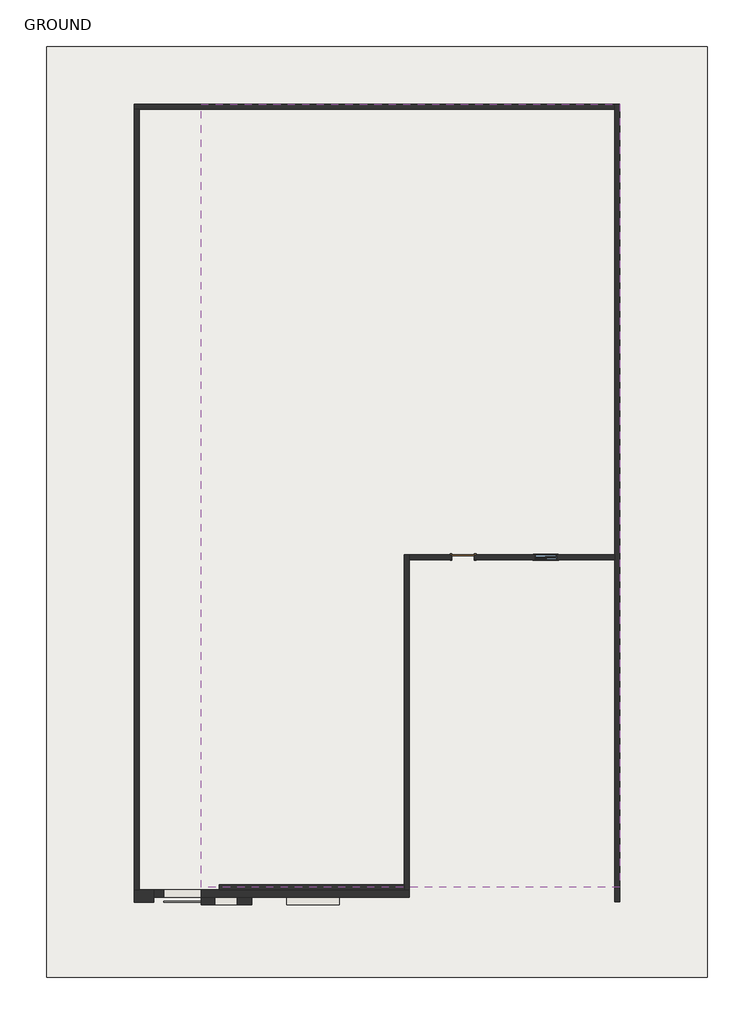
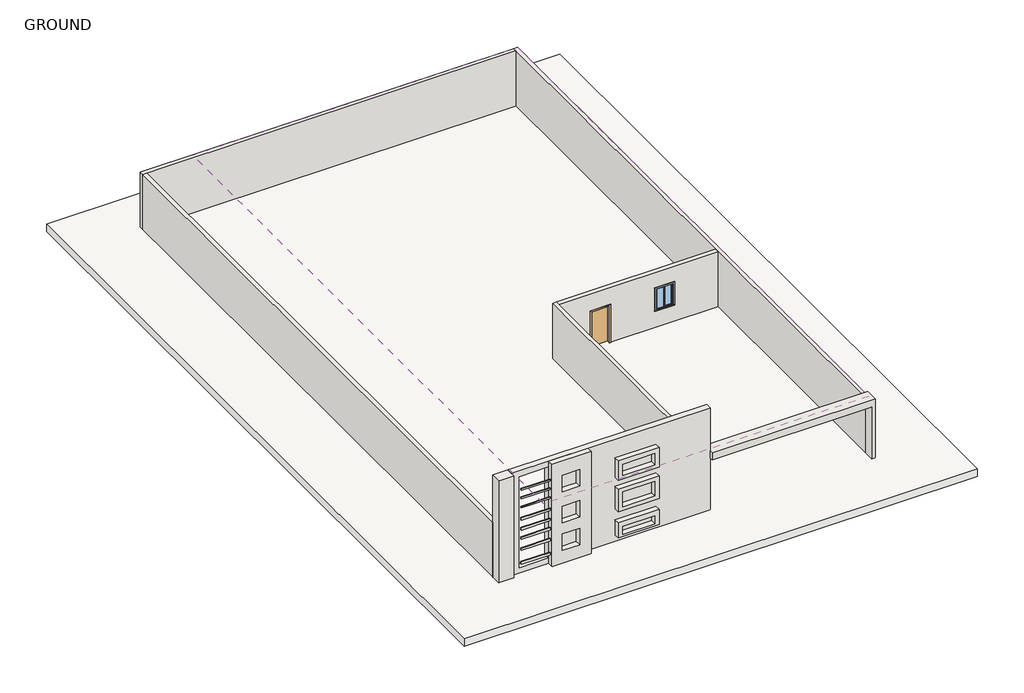
# One storey: 12 walls, 1 covering, 1 door, 1 slab, 1 window.
"""IFC4 building model written with IfcOpenShell, lengths in millimetres."""

from ifc_helpers import new_model, si_unit, frame, origin, origin_with_axes, place, context, project, spatial, polyline, outline, extrude, faceted_brep, transform, mapped, element, save
from components import m_single_flush_0915_x_2032mm_26613924, walls_2_walls_2_e7feafe1, walls_3_walls_3_a1481ceb, walls_4_walls_4_1aaea7ad, walls_5_walls_5_99fd860d, walls_6_walls_6_eefe2e9b, walls_7_walls_7_71d3a732, window_242facca

model = new_model("IFC4")

# Units and contexts
model_context = context("Model", 3, world=origin())
ifc_project = project(units=[si_unit("LENGTHUNIT", "METRE", prefix="MILLI")], contexts=[model_context])

# Site, building, storey
site = spatial("IfcSite", under=ifc_project)
building = spatial("IfcBuilding", under=site)
storey = spatial("IfcBuildingStorey", under=building, Name="GROUND", Elevation=0.0)

# Covering
placement = place(None, origin())
element("IfcCovering", 1, ObjectType="600 x 1200mm grid", at=placement, inside=storey, context=model_context, shape_type="SweptSolid", body=[
    extrude(outline(polyline([(-15779.6883357, -20030.9210337), (-15779.6883357, 11768.2789663), (1204.9616643, 11768.2789663), (1204.9616643, -20030.9210337), (-15779.6883357, -20030.9210337)])), frame((0.0, 0.0, 3048.0), z_axis=(0.0, 0.0, 1.0), x_axis=(1.0, 0.0, 0.0)), (0.0, 0.0, 1.0), 52.0),
])

# Door
m_single_flush_0915_x_2032mm_shape = m_single_flush_0915_x_2032mm_26613924(model_context)
element("IfcDoor", 2, ObjectType="M_Single-Flush : 0915 x 2032mm", at=placement, inside=storey, context=model_context, shape_type="MappedRepresentation", body=[
    mapped(m_single_flush_0915_x_2032mm_shape, transform((-5143.4383357, -6619.7210337, 0.0), x_axis=(-1.0, 0.0, 0.0), y_axis=(0.0, -1.0, 0.0), z_axis=(0.0, 0.0, 1.0))),
])

# Slab
element("IfcSlab", 3, ObjectType="Generic Floor - 400mm", at=placement, inside=storey, context=model_context, shape_type="SweptSolid", body=[
    extrude(outline(polyline([(4762.5616643, 14106.6789663), (4762.5616643, -23688.5210337), (-22059.8383357, -23688.5210337), (-22059.8383357, 14106.6789663), (4762.5616643, 14106.6789663)])), frame((0.0, 0.0, -400.0), z_axis=(0.0, 0.0, 1.0), x_axis=(1.0, 0.0, 0.0)), (0.0, 0.0, 1.0), 400.0),
])

# Walls
element("IfcWall", 4, ObjectType="Generic - 9\"", at=placement, inside=storey, context=model_context, shape_type="Brep", body=[
    faceted_brep([(-18502.2383357, 11568.2789663, 0.0), (-18302.2383357, 11568.2789663, 0.0), (1004.9616643, 11568.2789663, 0.0), (1004.9616643, 11568.2789663, 3048.0), (-18302.2383357, 11568.2789663, 3048.0), (-18502.2383357, 11568.2789663, 3048.0), (-18502.2383357, 11768.2789663, 0.0), (-18502.2383357, 11768.2789663, 3048.0), (1004.9616643, 11768.2789663, 3048.0), (1004.9616643, 11768.2789663, 0.0)], [[[0, 1, 2, 3, 4, 5]], [[6, 7, 8, 9]], [[2, 1, 0, 6, 9]], [[5, 4, 3, 8, 7]], [[0, 5, 7, 6]], [[3, 2, 9, 8]]]),
])
element("IfcWall", 5, ObjectType="Generic - 9\"", at=placement, inside=storey, context=model_context, shape_type="SweptSolid", body=[
    extrude(outline(polyline([(-18302.2383357, 11568.2789663), (-18302.2383357, -20130.9210337), (-18502.2383357, -20130.9210337), (-18502.2383357, 11568.2789663), (-18302.2383357, 11568.2789663)])), origin_with_axes(), (0.0, 0.0, 1.0), 3048.0),
])
element("IfcWall", 6, ObjectType="Generic - 9\"", at=placement, inside=storey, context=model_context, shape_type="SweptSolid", body=[
    extrude(outline(polyline([(-15049.4383357, -19930.9210337), (-7529.4383357, -19930.9210337), (-7529.4383357, -20130.9210337), (-15049.4383357, -20130.9210337), (-15049.4383357, -19930.9210337)])), origin_with_axes(), (0.0, 0.0, 1.0), 3048.0),
])
element("IfcWall", 7, ObjectType="Generic - 9\"", at=placement, inside=storey, context=model_context, shape_type="Brep", body=[
    faceted_brep([(1004.9616643, 11768.2789663, 0.0), (1004.9616643, 11568.2789663, 0.0), (1004.9616643, -6519.7210337, 0.0), (1004.9616643, -6719.7210337, 0.0), (1004.9616643, -20030.9210337, 0.0), (1004.9616643, -20030.9210337, 3048.0), (1004.9616643, -6719.7210337, 3048.0), (1004.9616643, -6519.7210337, 3048.0), (1004.9616643, 11568.2789663, 3048.0), (1004.9616643, 11768.2789663, 3048.0), (1204.9616643, 11768.2789663, 0.0), (1204.9616643, 11768.2789663, 3048.0), (1204.9616643, -20030.9210337, 3048.0), (1204.9616643, -20030.9210337, 0.0)], [[[0, 1, 2, 3, 4, 5, 6, 7, 8, 9]], [[10, 11, 12, 13]], [[4, 3, 2, 1, 0, 10, 13]], [[5, 4, 13, 12]], [[9, 8, 7, 6, 5, 12, 11]], [[0, 9, 11, 10]]]),
])
element("IfcWall", 8, ObjectType="Generic - 9\"", at=placement, inside=storey, context=model_context, shape_type="Brep", body=[
    faceted_brep([(-7329.4383357, -20130.9210337, 0.0), (-7329.4383357, -6719.7210337, 0.0), (-7329.4383357, -6519.7210337, 0.0), (-7329.4383357, -6519.7210337, 3048.0), (-7329.4383357, -6719.7210337, 3048.0), (-7329.4383357, -20130.9210337, 3048.0), (-7529.4383357, -20130.9210337, 0.0), (-7529.4383357, -20130.9210337, 3048.0), (-7529.4383357, -19930.9210337, 3048.0), (-7529.4383357, -6519.7210337, 3048.0), (-7529.4383357, -6519.7210337, 0.0), (-7529.4383357, -19930.9210337, 0.0)], [[[0, 1, 2, 3, 4, 5]], [[6, 7, 8, 9, 10, 11]], [[2, 1, 0, 6, 11, 10]], [[5, 4, 3, 9, 8, 7]], [[3, 2, 10, 9]], [[0, 5, 7, 6]]]),
])
element("IfcWall", 9, ObjectType="Generic - 9\"", at=placement, inside=storey, context=model_context, shape_type="SweptSolid", body=[
    extrude(outline(polyline([(0.0, -7329.4383357), (0.0, -5600.9383357), (2032.0, -5600.9383357), (2032.0, -4685.9383357), (0.0, -4685.9383357), (0.0, 1004.9616643), (3048.0, 1004.9616643), (3048.0, -7329.4383357), (0.0, -7329.4383357)]), holes=[polyline([(2133.6, -2247.8383357), (2133.6, -1333.4383357), (914.4, -1333.4383357), (914.4, -2247.8383357), (2133.6, -2247.8383357)])]), frame((0.0, -6719.7210337, 0.0), z_axis=(0.0, 1.0, 0.0), x_axis=(0.0, 0.0, 1.0)), (0.0, 0.0, 1.0), 200.0),
])
walls_2_walls_2_shape = walls_2_walls_2_e7feafe1(model_context)
element("IfcWall", 10, ObjectType="Walls 2 : Walls 2", at=placement, inside=storey, context=model_context, shape_type="MappedRepresentation", body=[
    mapped(walls_2_walls_2_shape, transform((0.0, 0.0, 0.0), x_axis=(1.0, 0.0, 0.0), y_axis=(0.0, 1.0, 0.0), z_axis=(0.0, 0.0, 1.0))),
])
walls_3_walls_3_shape = walls_3_walls_3_a1481ceb(model_context)
element("IfcWall", 11, ObjectType="Walls 3 : Walls 3", at=placement, inside=storey, context=model_context, shape_type="MappedRepresentation", body=[
    mapped(walls_3_walls_3_shape, transform((0.0, 0.0, 0.0), x_axis=(1.0, 0.0, 0.0), y_axis=(0.0, 1.0, 0.0), z_axis=(0.0, 0.0, 1.0))),
])
walls_4_walls_4_shape = walls_4_walls_4_1aaea7ad(model_context)
element("IfcWall", 12, ObjectType="Walls 4 : Walls 4", at=placement, inside=storey, context=model_context, shape_type="MappedRepresentation", body=[
    mapped(walls_4_walls_4_shape, transform((0.0, 0.0, 0.0), x_axis=(1.0, 0.0, 0.0), y_axis=(0.0, 1.0, 0.0), z_axis=(0.0, 0.0, 1.0))),
])
walls_5_walls_5_shape = walls_5_walls_5_99fd860d(model_context)
element("IfcWall", 13, ObjectType="Walls 5 : Walls 5", at=placement, inside=storey, context=model_context, shape_type="MappedRepresentation", body=[
    mapped(walls_5_walls_5_shape, transform((0.0, 0.0, 0.0), x_axis=(1.0, 0.0, 0.0), y_axis=(0.0, 1.0, 0.0), z_axis=(0.0, 0.0, 1.0))),
])
walls_6_walls_6_shape = walls_6_walls_6_eefe2e9b(model_context)
element("IfcWall", 14, ObjectType="Walls 6 : Walls 6", at=placement, inside=storey, context=model_context, shape_type="MappedRepresentation", body=[
    mapped(walls_6_walls_6_shape, transform((0.0, 0.0, 0.0), x_axis=(1.0, 0.0, 0.0), y_axis=(0.0, 1.0, 0.0), z_axis=(0.0, 0.0, 1.0))),
])
walls_7_walls_7_shape = walls_7_walls_7_71d3a732(model_context)
element("IfcWall", 15, ObjectType="Walls 7 : Walls 7", at=placement, inside=storey, context=model_context, shape_type="MappedRepresentation", body=[
    mapped(walls_7_walls_7_shape, transform((0.0, 0.0, 0.0), x_axis=(1.0, 0.0, 0.0), y_axis=(0.0, 1.0, 0.0), z_axis=(0.0, 0.0, 1.0))),
])

# Window
window_shape = window_242facca(model_context)
element("IfcWindow", 16, ObjectType="Slider with Trim : 36\" x 48\"", at=placement, inside=storey, context=model_context, shape_type="MappedRepresentation", body=[
    mapped(window_shape, transform((-1790.6383357, -6619.7210337, 0.0), x_axis=(-1.0, 0.0, 0.0), y_axis=(0.0, -1.0, 0.0), z_axis=(0.0, 0.0, 1.0))),
])

save(model, "model.ifc")

# Revit data of these elements
# Type "600 x 1200mm grid"
#   built-in parameter 1002203 = 1 (stored number, unit not read)
#   built-in parameter 1002202 = 1 (stored number, unit not read)
#   Layers, outside or top first: 0' - 1.41732" "Default" (function 1); 0' - 0.62992" "Ceiling Tile 600 x 1200" (function 5)
# Type "M_Single-Flush : 0915 x 2032mm"
#   Type Mark = "20"
#   Thickness = 0' - 2.00787"
#   Height = 6' - 8"
#   Trim Projection Ext = 0' - 0.98425"
#   Trim Projection Int = 0' - 0.98425"
#   Trim Width = 0' - 2.99213"
#   Width = 3' - 0.02362"
#   Door Material = Door - Panel
#   Frame Material = Door - Frame
#   Function = (empty or 0)
#   Wall Closure = (empty or 0)
# Type "Generic Floor - 400mm"
#   Function = 0
#   Layers, outside or top first: 1' - 3.74803" no material (function 1)
# Type "Generic - 9\""
#   Layers, outside or top first: 0' - 7.87402" no material (function 1)
# Type "Slider with Trim : 36\" x 48\""
#   Type Mark = "19"
#   Construction Type Id = "GSP4R"
#   Assembly Code = "B2020100"
#   Analytic Construction = "1/8 in Pilkington single glazing"
#   Visual Light Transmittance = 0.9
#   Solar Heat Gain Coefficient = 0.78
#   Heat Transfer Coefficient (U) = 3.6886 W/(m²·K)
#   Height = 4' - 0"
#   Default Sill Height = 3' - 0"
#   Trim Projection - Ext. = 0' - 0 3/4"
#   Trim Projection - Int. = 0' - 0 3/4"
#   Trim Width - Exterior = 0' - 3 1/2"
#   Trim Width - Interior = 0' - 3 1/2"
#   Width = 3' - 0"
#   Window Inset = 0' - 0 3/4"
#   Define Thermal Properties by = 1
#   Glass Pane Material = Glass
#   Sash Material = Sash
#   Trim Exterior Material = Trim
#   Trim Interior Material = Trim
#   Wall Closure = (empty or 0)
# Element 1 (IfcCovering, "600 x 1200mm grid")
#   Height Offset From Level = 10' - 0"
#   Phase Created = New Construction
#   Materials on its faces: "Ceiling Tile 600 x 1200", "Default"
# Element 2 (IfcDoor, "M_Single-Flush : 0915 x 2032mm")
#   Phase Created = New Construction
#   Materials on its faces: "Door - Frame", "Door - Panel"
# Element 3 (IfcSlab, "Generic Floor - 400mm")
#   Height Offset From Level = 0' - 0"
#   Phase Created = New Construction
#   Materials on its faces: "Default Roof"
# Elements 4, 5, 6, 7, 8, 9 (IfcWall, "Generic - 9\"")
#   Top Offset = 0' - 0"
#   Base Offset = 0' - 0"
#   Unconnected Height = 10' - 0"
#   wall height = 10' - 0"
#   Phase Created = New Construction
#   Base Constraint = GROUND
#   Materials on its faces: "Default Wall"
# Element 10 (IfcWall, "Walls 2 : Walls 2")
#   Phase Created = New Construction
#   Materials on its faces: "Default Wall"
# Element 11 (IfcWall, "Walls 3 : Walls 3")
#   Phase Created = New Construction
#   Materials on its faces: "Default Wall"
# Element 12 (IfcWall, "Walls 4 : Walls 4")
#   Phase Created = New Construction
#   Materials on its faces: "Default Wall"
# Element 13 (IfcWall, "Walls 5 : Walls 5")
#   Phase Created = New Construction
#   Materials on its faces: "Default Wall"
# Element 14 (IfcWall, "Walls 6 : Walls 6")
#   Phase Created = New Construction
#   Materials on its faces: "Default Wall"
# Element 15 (IfcWall, "Walls 7 : Walls 7")
#   Phase Created = New Construction
#   Materials on its faces: "Default Wall"
# Element 16 (IfcWindow, "Slider with Trim : 36\" x 48\"")
#   Mark = "6"
#   Phase Created = New Construction
#   Materials on its faces: "Sash", "Trim", "Glass"
# Materials
#   "Default": colour RGB 80 80 80, transparency 0
#   "Ceiling Tile 600 x 1200": class "Generic", colour RGB 179 178 175, transparency 0, Description = "Acoustic ceiling tile", Cost = 0
#   "Door - Panel": class "Wood", colour RGB 114 82 51, transparency 0
#   "Door - Frame": colour RGB 153 76 43, transparency 0
#   "Glass": class "Glass", colour RGB 218 227 224, transparency 0.85, Description = "Soda Lime Glass", Cost = 0
#   "Sash": class "Wood", colour RGB 136 99 55, transparency 0
#   "Trim": class "Wood", colour RGB 224 178 126, transparency 0
#   "Default Roof": colour RGB 80 80 80, transparency 0
#   "Default Wall": colour RGB 80 80 80, transparency 0
